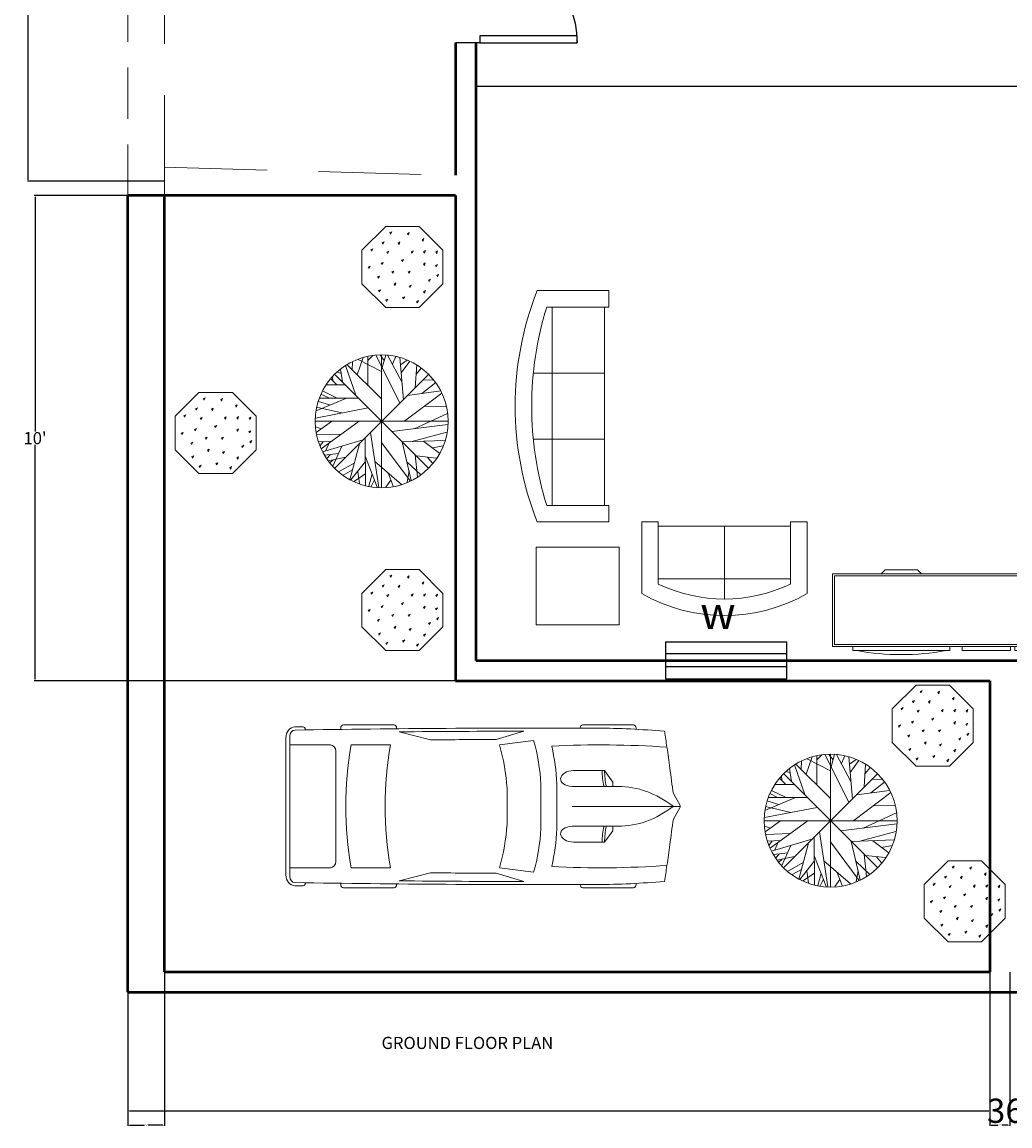
# Model space of a CAD drawing. Units: inches. Extents: x -10 to 557, y -66 to 886.
# Tile 1 of 6: x -3 to 241, y -66 to 207. Entities that reach past the tile are written whole.
import ezdxf

# ---------------------------------------------------------------- set-up
doc = ezdxf.new("R2010")
doc.units = ezdxf.units.IN
doc.header["$MEASUREMENT"] = 0
doc.linetypes.add('DASHED', pattern=[19.05, 12.7, -6.35])
for name, color, linetype, lineweight in [('A-ANNO-DIMS', 2, 'Continuous', 18), ('A-ANNO-TEXT', 7, 'Continuous', 18), ('A-DOOR', 4, 'Continuous', 25), ('A-EQPM', 9, 'Continuous', 18), ('A-FURN', 8, 'Continuous', 18), ('A-GLAZ', 4, 'Continuous', 25), ('A-WALL', 7, 'Continuous', 50), ('A-WALL-OVHD', 8, 'DASHED', 18), ('L-PLNT', 3, 'Continuous', 18)]:
    doc.layers.add(name, color=color, linetype=linetype, lineweight=lineweight)
doc.styles.get("Standard").update_dxf_attribs({"font": 'arial.ttf'})
doc.dimstyles.get("Standard").update_dxf_attribs({"dimtxt": 0.3, "dimasz": 0.4, "dimexe": 0.18, "dimexo": 0.0625, "dimgap": 0.09, "dimtad": 0, "dimtih": 1, "dimtoh": 1, "dimdec": 0, "dimrnd": 8, "dimzin": 0, "dimdsep": 46, "dimlunit": 3, "dimtxsty": 'Standard', "dimcen": 0.09, "dimadec": 0, "dimazin": 0, "dimtfac": 1, "dimtdec": 0, "dimtofl": 0, "dimtmove": 0, "dimatfit": 3, "dimfxl": 1, "dimtolj": 1, "dimtzin": 0, "dimarcsym": 0})

# ---------------------------------------------------------------- blocks, each defined once
blk = doc.blocks.new('*U33')
for p, q in [((0, 0), (0, -6)), ((24, 0), (24, -6))]:
    blk.add_line(p, q)
blk.add_lwpolyline([(0, 0), (0, 24), (1.75, 24), (1.75, 0)], close=True)
blk.add_arc((0, 0), 24, 0, 90)
blk = doc.blocks.new('Sofa - Roundback 7 ft.')
for p, q in [((-12.00002, -32.4421), (-12.00003, -6.5971)), ((11.99997, -32.4421), (11.99998, -6.5971)), ((-36.000027, -34), (-36.000027, -11.4696)), ((35.99998, -34), (35.99998, -11.4696)), ((-35.999844, -13.3819), (35.9998, -13.3819)), ((-36.000027, -32.4421), (35.99998, -32.4421))]:
    blk.add_line(p, q)
for points in [[(-36.000027, -34), (-42.000027, -34), (-42.000027, -8)], [(41.99998, -8), (41.99998, -34), (35.99998, -34)]]:
    blk.add_lwpolyline(points)
for centre, radius, start, end in [((0, -114.25), 114.25, 68.43141, 111.5686), ((-0.00001, -127.1968), 121.1968, 72.72033, 107.2797)]:
    blk.add_arc(centre, radius, start, end)
blk = doc.blocks.new('Sofa - Roundback Loveseat 5 ft.')
for p, q in [((0, -32.44198), (0, -5.99998)), ((-24, -33.99998), (-24, -11.46958)), ((24.00004, -33.99998), (24.00004, -11.46958)), ((-23.9998, -13.38178), (23.99986, -13.38178)), ((-24, -32.44198), (24.00004, -32.44198))]:
    blk.add_line(p, q)
for points in [[(-24, -33.99998), (-30, -33.99998), (-30, -7.99998)], [(30.00004, -7.99998), (30.00004, -33.99998), (24.00004, -33.99998)]]:
    blk.add_lwpolyline(points)
for centre, radius, start, end in [((0, -60.24998), 60.24998, 60.13715, 119.8628), ((0, -61.38438), 55.38444, 64.32083, 115.6792)]:
    blk.add_arc(centre, radius, start, end)
blk = doc.blocks.new('*U36')
for p, q in [((21.1, 37.41), (21.1, 36.83)), ((46.55, 38.89), (22.35, 38.89)), ((47.8, 37.39), (47.8, 37.41)), ((135.45, 37.07), (135.45, 37.41)), ((136.7, 38.89), (160.9, 38.89)), ((162.15, 37.41), (162.15, 36.77)), ((87.99, 31.87), (74.76, 35.92)), ((134.31, 35.6), (119.29, 31.78)), ((186.47, -33.5), (186.47, 33.5)), ((188.4, -32.76), (188.4, 32.76)), ((70.03, 31.54), (86.41, 29.35)), ((138.42, 29.35), (157.25, 29.35)), ((164.52, 26.39), (164.52, -26.39)), ((186.47, 29.35), (167.01, 29.35)), ((32.27, 11.63), (36.13, 17.17)), ((36.13, 17.17), (50.94, 17.17)), ((32.12, 9.51), (32.12, 11.15)), ((58.92, -10.77), (58.92, 10.77)), ((3.27, 6.13), (0.1, 0.41)), ((29.77, 9.51), (51.68, 9.51)), ((66.55, -10.53), (66.55, 10.53)), ((82.74, 8.5), (82.74, -8.5)), ((186.47, -10.53), (186.47, 10.53)), ((0, 0), (51.68, 0)), ((0.1, -0.41), (3.27, -6.13)), ((29.77, -9.51), (51.68, -9.51)), ((32.12, -9.51), (32.12, -11.15)), ((32.27, -11.63), (36.13, -17.17)), ((36.13, -17.17), (50.94, -17.17)), ((86.41, -29.35), (70.03, -31.54)), ((157.25, -29.35), (138.42, -29.35)), ((167.01, -29.35), (186.47, -29.35)), ((21.1, -37.41), (21.1, -36.83)), ((87.99, -31.87), (74.76, -35.92)), ((134.31, -35.6), (119.29, -31.78)), ((162.15, -37.41), (162.15, -36.77)), ((46.55, -38.89), (22.35, -38.89)), ((47.8, -37.39), (47.8, -37.41)), ((135.45, -37.07), (135.45, -37.41)), ((136.7, -38.89), (160.9, -38.89))]:
    blk.add_line(p, q)
for centre, major_axis, ratio, start_param, end_param in [((41.19, -490.86), (0, 528.23), 0.842304, 0.00281, 0.075598), ((22.35, 37.41), (0, -1.48), 0.842304, 3.141593, 4.712389), ((64.48, -10555.62), (0, 10593.03), 0.842304, -0.013397, 0.002797), ((46.55, 37.41), (0, 1.48), 0.842304, -1.570796, 0), ((136.7, 37.41), (0, -1.48), 0.842304, 3.141593, 4.712389), ((160.9, 37.41), (0, 1.48), 0.842304, -1.570796, 0), ((180.63, 35.84), (0, 2.22), 0.842304, -0.013017, 1.249894), ((64.48, -10556.36), (0, 10595.31), 0.842304, -0.013397, -0.013017), ((183.98, 32.76), (0, -5.25), 0.842304, 1.570796, 3.128196), ((266.03, -27.52), (0, 313.31), 0.842304, 1.367076, 1.39176), ((64.48, -10555.62), (0, -10591.55), 0.842304, 3.133765, 3.140441), ((95.79, -3666.35), (0, -3698.24), 0.842304, 3.134049, 3.144098), ((183.98, 33.5), (0, -2.96), 0.842304, 1.570796, 3.128196), ((259.18, -27.52), (0, -305.3), 0.842304, 4.528606, 4.561838), ((37.47, -593.96), (0, -623.33), 0.842304, 3.096046, 3.200911), ((134.4, 5.39), (0, -89.78), 0.842304, 4.449482, 4.652344), ((135.29, 5.39), (0, 81.77), 0.842304, 1.245306, 1.50788), ((149.6, 2.8), (0, -79.58), 0.842304, 4.372215, 4.640744), ((17.08, 0), (0, 147.02), 0.842304, 4.511394, 4.913384), ((35.91, 0), (0, 147.02), 0.842304, 4.511394, 4.913384), ((167.01, 26.39), (0, 2.96), 0.842304, 0, 1.570796), ((-204.49, 52.4), (0, -250.96), 0.842304, 1.385369, 1.434372), ((13.04, 17.01), (0, 27.42), 0.842304, 4.435146, 4.718221), ((14.2, 17.01), (0, 27.42), 0.842304, 4.435146, 4.718221), ((50.79, 13.34), (6.34, -0.36), 0.603834, -1.395552, 1.581315), ((32.75, 11.15), (0, 0.74), 0.842304, 0.879714, 1.570796), ((29.77, -46.66), (0, 56.17), 0.842304, 0, 0.590319), ((0.62, 0), (0, -0.74), 0.842304, 4.131459, 5.293319), ((29.77, 46.66), (0, 56.17), 0.842304, 2.551274, 3.141593), ((-204.49, -52.4), (0, 250.96), 0.842304, -1.434372, -1.385369), ((13.04, -17.01), (0, -27.42), 0.842304, 1.564964, 1.848039), ((14.2, -17.01), (0, -27.42), 0.842304, 1.564964, 1.848039), ((135.29, -5.39), (0, -81.77), 0.842304, -1.50788, -1.245306), ((149.6, -2.8), (0, -79.58), 0.842304, -1.499151, -1.230623), ((32.75, -11.15), (0, -0.74), 0.842304, 4.712389, 5.403472), ((134.4, -5.39), (0, -89.78), 0.842304, -1.510751, -1.307889), ((259.18, 27.52), (0, 305.3), 0.842304, 1.721348, 1.754579), ((266.03, 27.52), (0, 313.31), 0.842304, 1.749832, 1.774517), ((37.47, 593.96), (0, -623.33), 0.842304, -0.059319, 0.045547), ((167.01, -26.39), (0, -2.96), 0.842304, 4.712389, 6.283185), ((41.19, 490.86), (0, -528.23), 0.842304, -0.075598, -0.00281), ((64.48, 10555.62), (0, 10593.03), 0.842304, 3.138796, 3.15499), ((64.48, 10555.62), (0, -10591.55), 0.842304, 0.001152, 0.007828), ((95.79, 3666.35), (0, -3698.24), 0.842304, -0.002505, 0.007544), ((180.63, -35.84), (0, -2.22), 0.842304, -1.249894, 0.013017), ((183.98, -33.5), (0, 2.96), 0.842304, 3.15499, 4.712389), ((183.98, -32.76), (0, -5.25), 0.842304, 0.013397, 1.570796), ((22.35, -37.41), (0, 1.48), 0.842304, 1.570796, 3.141593), ((46.55, -37.41), (0, -1.48), 0.842304, 0, 1.570796), ((136.7, -37.41), (0, -1.48), 0.842304, -1.570796, 0), ((160.9, -37.41), (0, 1.48), 0.842304, 3.141593, 4.712389), ((64.48, 10556.36), (0, 10595.31), 0.842304, 3.15461, 3.15499)]:
    blk.add_ellipse(centre, major_axis=major_axis, ratio=ratio, start_param=start_param, end_param=end_param)
at = {"extrusion": (0, 0, -1)}
blk.add_ellipse((50.79, -13.34), major_axis=(6.34, 0.36), ratio=0.603834, start_param=-1.395552, end_param=1.581315, dxfattribs=at)
blk = doc.blocks.new('*D42')
at = {"layer": 'A-ANNO-DIMS', "color": 0, "lineweight": -2, "ltscale": 2, "transparency": 16777216}
for p, q in [((31.91, 265.32), (-1.86, 265.32)), ((-1.68, 264.92), (-1.68, 218.2)), ((-1.68, 168.23), (-1.68, 214.95)), ((31.91, 167.83), (-1.86, 167.83))]:
    blk.add_line(p, q, dxfattribs=at)
at = {"layer": 'A-ANNO-DIMS', "color": 0, "ltscale": 2, "transparency": 16777216}
for points in [[(-1.75, 264.92), (-1.61, 264.92), (-1.68, 265.32)], [(-1.75, 168.23), (-1.61, 168.23), (-1.68, 167.83)]]:
    blk.add_solid(points, dxfattribs=at)
at = {"layer": 'Defpoints', "color": 0, "ltscale": 2, "transparency": 16777216}
for p in [(31.97, 265.32), (-1.68, 167.83), (31.97, 167.83)]:
    blk.add_point(p, dxfattribs=at)
at = {"layer": 'A-ANNO-DIMS', "color": 0, "ltscale": 2, "transparency": 16777216, "insert": (-1.68, 216.57), "char_height": 0.3, "attachment_point": 5}
blk.add_mtext("\\A1;{\\H10x;8'}", dxfattribs=at)
blk = doc.blocks.new('*D43')
at = {"layer": 'A-ANNO-DIMS', "color": 0, "lineweight": -2, "ltscale": 2, "transparency": 16777216}
for p, q in [((103.91, 164.32), (-0.17, 164.32)), ((0.01, 163.92), (0.01, 105.94)), ((0.01, 44.72), (0.01, 102.7)), ((103.91, 44.32), (-0.17, 44.32))]:
    blk.add_line(p, q, dxfattribs=at)
at = {"layer": 'A-ANNO-DIMS', "color": 0, "ltscale": 2, "transparency": 16777216}
for points in [[(-0.06, 163.92), (0.08, 163.92), (0.01, 164.32)], [(-0.06, 44.72), (0.08, 44.72), (0.01, 44.32)]]:
    blk.add_solid(points, dxfattribs=at)
at = {"layer": 'Defpoints', "color": 0, "ltscale": 2, "transparency": 16777216}
for p in [(103.97, 164.32), (0.01, 44.32), (103.97, 44.32)]:
    blk.add_point(p, dxfattribs=at)
at = {"layer": 'A-ANNO-DIMS', "color": 0, "ltscale": 2, "transparency": 16777216, "insert": (0.01, 104.32), "char_height": 0.3, "attachment_point": 5}
blk.add_mtext("\\A1;{\\H10x;10'}", dxfattribs=at)
blk = doc.blocks.new('*D49')
at = {"layer": 'A-ANNO-DIMS', "color": 0, "lineweight": -2, "ltscale": 2, "transparency": 16777216}
for p, q in [((108.97, 177.7), (108.97, 191.53)), ((109.37, 191.35), (274.2, 191.35)), ((449.57, 191.35), (284.74, 191.35)), ((449.97, 177.7), (449.97, 191.53))]:
    blk.add_line(p, q, dxfattribs=at)
at = {"layer": 'A-ANNO-DIMS', "color": 0, "ltscale": 2, "transparency": 16777216}
for points in [[(109.37, 191.42), (109.37, 191.28), (108.97, 191.35)], [(449.57, 191.42), (449.57, 191.28), (449.97, 191.35)]]:
    blk.add_solid(points, dxfattribs=at)
at = {"layer": 'Defpoints', "color": 0, "ltscale": 2, "transparency": 16777216}
for p in [(449.97, 191.35), (108.97, 177.64), (449.97, 177.64)]:
    blk.add_point(p, dxfattribs=at)
at = {"layer": 'A-ANNO-DIMS', "color": 0, "ltscale": 2, "transparency": 16777216, "insert": (279.47, 191.35), "char_height": 0.3, "attachment_point": 5}
blk.add_mtext('\\A1;{\\H10x;28\'-8"}', dxfattribs=at)
blk = doc.blocks.new('Stepping Stone - hexagonal')
for p, q in [((-5.1, 10.07), (-10.96, 4.2)), ((3.2, 10.07), (-5.1, 10.07)), ((-3.56, 8.74), (-4.06, 8.54)), ((-4.06, 8.54), (-3.91, 8.2)), ((-3.91, 8.2), (-3.56, 8.74)), ((0.7, 8.56), (0.27, 8.26)), ((0.27, 8.26), (0.5, 7.96)), ((0.5, 7.96), (0.7, 8.56)), ((9.06, 4.2), (3.2, 10.07)), ((-5.45, 6.27), (-5.95, 6.07)), ((-5.95, 6.07), (-5.79, 5.73)), ((-5.79, 5.73), (-5.45, 6.27)), ((-1.57, 6.24), (-2, 5.93)), ((-2, 5.93), (-1.77, 5.63)), ((-1.77, 5.63), (-1.57, 6.24)), ((4.33, 7.05), (3.9, 6.74)), ((3.9, 6.74), (4.13, 6.45)), ((4.13, 6.45), (4.33, 7.05)), ((-10.96, 4.2), (-10.96, -4.09)), ((-8.31, 4.52), (-8.81, 4.32)), ((-8.81, 4.32), (-8.65, 3.98)), ((-8.65, 3.98), (-8.31, 4.52)), ((-4.32, 3.92), (-4.82, 3.72)), ((-4.82, 3.72), (-4.67, 3.38)), ((-4.67, 3.38), (-4.32, 3.92)), ((1.65, 4.08), (1.22, 3.77)), ((1.22, 3.77), (1.45, 3.48)), ((1.45, 3.48), (1.65, 4.08)), ((4.71, 4.1), (4.27, 3.8)), ((4.27, 3.8), (4.5, 3.5)), ((4.5, 3.5), (4.71, 4.1)), ((7.74, 4.01), (7.3, 3.7)), ((7.3, 3.7), (7.53, 3.41)), ((7.53, 3.41), (7.74, 4.01)), ((9.06, -4.09), (9.06, 4.2)), ((-8.97, 0.22), (-9.47, 0.02)), ((-9.47, 0.02), (-9.31, -0.32)), ((-9.31, -0.32), (-8.97, 0.22)), ((-5.72, 1.16), (-6.22, 0.96)), ((-6.22, 0.96), (-6.07, 0.63)), ((-6.07, 0.63), (-5.72, 1.16)), ((-0.72, 1.92), (-1.22, 1.73)), ((-1.22, 1.73), (-1.07, 1.39)), ((-1.07, 1.39), (-0.72, 1.92)), ((4.67, 1.05), (4.23, 0.74)), ((4.23, 0.74), (4.46, 0.44)), ((4.46, 0.44), (4.67, 1.05)), ((7.72, 0.63), (7.23, 0.43)), ((7.23, 0.43), (7.38, 0.09)), ((7.38, 0.09), (7.72, 0.63)), ((-6.63, -2.22), (-7.13, -2.42)), ((-7.13, -2.42), (-6.97, -2.76)), ((-6.97, -2.76), (-6.63, -2.22)), ((-3.1, -0.96), (-3.6, -1.16)), ((-3.6, -1.16), (-3.44, -1.5)), ((-3.44, -1.5), (-3.1, -0.96)), ((0.94, -0.97), (0.45, -1.17)), ((0.45, -1.17), (0.6, -1.51)), ((0.6, -1.51), (0.94, -0.97)), ((7.94, -1.78), (7.5, -2.09)), ((7.5, -2.09), (7.73, -2.38)), ((7.73, -2.38), (7.94, -1.78)), ((-10.96, -4.09), (-5.1, -9.96)), ((-2.57, -3.91), (-3, -4.22)), ((-3, -4.22), (-2.77, -4.51)), ((-2.77, -4.51), (-2.57, -3.91)), ((1.22, -4.48), (0.72, -4.68)), ((0.72, -4.68), (0.88, -5.02)), ((0.88, -5.02), (1.22, -4.48)), ((3.2, -9.96), (9.06, -4.09)), ((5.96, -2.99), (5.47, -3.18)), ((5.47, -3.18), (5.62, -3.52)), ((5.62, -3.52), (5.96, -2.99)), ((-6.38, -5.59), (-6.87, -5.79)), ((-6.87, -5.79), (-6.72, -6.13)), ((-6.72, -6.13), (-6.38, -5.59)), ((-4.59, -7.91), (-5.08, -8.11)), ((-5.08, -8.11), (-4.93, -8.45)), ((-4.93, -8.45), (-4.59, -7.91)), ((-0.41, -7.32), (-0.91, -7.51)), ((-0.91, -7.51), (-0.76, -7.85)), ((-0.76, -7.85), (-0.41, -7.32)), ((4.7, -5.8), (4.26, -6.11)), ((4.26, -6.11), (4.49, -6.4)), ((4.49, -6.4), (4.7, -5.8)), ((-5.1, -9.96), (3.2, -9.96)), ((2.97, -8.26), (2.54, -8.57)), ((2.54, -8.57), (2.77, -8.86)), ((2.77, -8.86), (2.97, -8.26))]:
    blk.add_line(p, q)
blk = doc.blocks.new('Tree - deciduous plan')
for p, q in [((2.426, 54.9406), (-1.4472, 59.9056)), ((0, 59.9996), (0, -60)), ((-32.6092, 50.4264), (-23.2782, 23.5674)), ((-31.2008, 51.1035), (-0.2149, 20.1818)), ((-26.4472, 46.5894), (-26.2712, 53.8116)), ((-22.0458, 42.0753), (-16.5881, 57.6486)), ((-21.1656, 55.8436), (-0.0388, 45.0094)), ((-12.5388, 54.9406), (-7.9613, 59.4546)), ((-12.3627, 32.1443), (-12.5388, 58.7776)), ((-5.3205, 59.6806), (16.5105, 16.7963)), ((0.4894, 48.6208), (3.6584, 59.6806)), ((18.2711, 35.5298), (5.419, 59.6806)), ((9.8203, 51.5549), (12.8133, 58.5516)), ((19.6795, 19.5047), (16.3344, 57.6486)), ((17.0387, 51.1035), (23.2006, 55.1666)), ((17.7429, 43.6552), (25.4894, 54.2636)), ((31.6513, 50.8778), (30.2429, 30.5643)), ((-43.8768, 36.4326), (-44.405, 40.2696)), ((42, 42), (-42, -42)), ((42, -42), (-42, 42)), ((-40.1797, 44.558), (-36.4825, 43.2038)), ((-37.0107, 47.0408), (-35.25, 35.5298)), ((31.1232, 42.5267), (35.8767, 48.1693)), ((-49.8627, 32.8214), (-32.7853, 32.8214)), ((-45.8134, 38.2383), (-40.5318, 33.0471)), ((36.2288, 25.1474), (48.9049, 35.0784)), ((37.1091, 37.1098), (46.6161, 37.5612)), ((-32.2571, 20.6333), (-59.1937, 9.348)), ((-56.0247, 20.859), (-20.8134, 20.859)), ((-54.7923, 24.4702), (-47.75, 21.0847)), ((-53.2078, 27.4044), (-40.1797, 20.859)), ((54.3626, 25.3731), (20.9119, 0.3198)), ((23.3767, 23.3417), (53.3063, 27.4044)), ((-59.7219, 2.8025), (-12.0106, 12.0565)), ((-58.6656, 12.7336), (-35.9543, 7.5424)), ((-57.081, 17.9248), (-47.0458, 14.7649)), ((38.5175, 13.4107), (58.2359, 13.6364)), ((-54.6162, -24.7335), (-20.2853, 0.0941)), ((29.3626, -6.6771), (59.4682, 7.091)), ((-60, 0), (60, 0)), ((-59.7219, -4.8714), (-54.2641, -6.6771)), ((-45.2853, -0.1316), (-59.0177, -10.0627)), ((9.2922, -9.1598), (59.6443, -2.8401)), ((26.3697, -18.4138), (58.9401, -9.8369)), ((-58.4895, -12.3197), (-36.4825, -11.6426)), ((-57.081, -18.4138), (-45.2853, -17.9624)), ((-52.6797, -18.188), (-55.4966, -22.0251)), ((-53.2078, -27.442), (-16.7641, -16.6081)), ((-47.2219, -19.3166), (-50.2148, -26.3135)), ((-14.8275, -15.0282), (-14.6515, -57.6865)), ((-10.074, -10.0627), (-2.5036, -59.7178)), ((-0.0388, -19.0909), (25.8415, -53.8495)), ((18.6232, -18.6394), (26.7218, -53.3981)), ((18.7992, -18.6394), (57.3556, -17.2853)), ((38.1654, -18.188), (52.426, -29.0219)), ((-38.9472, -29.0219), (-51.4472, -30.6018)), ((-35.9543, -22.4765), (-44.0529, -40.5329)), ((-19.9331, -20.2194), (-28.5599, -52.721)), ((45.9119, -24.0564), (55.595, -22.2508)), ((-46.5177, -30.1504), (-49.5106, -33.536)), ((-32.4331, -32.4075), (-48.1021, -35.5674)), ((-43.7008, -34.6645), (-46.6937, -37.373)), ((-24.6867, -37.8244), (-38.7712, -45.7241)), ((-14.6515, -36.2445), (-27.6797, -52.9467)), ((-14.6515, -32.1818), (-3.912, -59.4922)), ((-6.2008, -36.2445), (17.919, -57.0094)), ((22.8485, -36.4702), (35.3485, -48.4326)), ((30.419, -30.1504), (32.3556, -50.0125)), ((31.4753, -31.279), (49.6091, -33.3103)), ((41.5105, -32.6332), (46.088, -38.0501)), ((-26.2712, -43.9185), (-34.7219, -48.6583)), ((-14.6515, -47.3041), (-25.0388, -54.3009)), ((-21.5177, -45.4984), (-19.9331, -56.1065)), ((-8.4895, -47.5298), (-11.4825, -58.5893)), ((5.9471, -46.6269), (10.5246, -58.5893)), ((24.7852, -44.8213), (23.0246, -54.978)), ((-6.3768, -52.721), (-9.3698, -58.815)), ((8.4119, -53.1724), (3.8344, -59.4922))]:
    blk.add_line(p, q)
blk.add_circle((0, 0), 60)
blk = doc.blocks.new('Entertainment Center')
for p, q in [((-4, 0), (-5, -1)), ((4, 0), (-4, 0)), ((5, -1), (4, 0)), ((-17, -19), (-17, -1)), ((-17, -1), (43, -1)), ((-16.5, -18.5), (-16.5, -1.5)), ((-16.5, -1.5), (42.5, -1.5)), ((42.5, -1.5), (42.5, -18.5)), ((43, -1), (43, -19)), ((43, -19), (-17, -19)), ((42.5, -18.5), (-16.5, -18.5)), ((-12, -20), (-12, -19)), ((12, -19), (12, -20)), ((15, -20), (15, -19)), ((27, -19), (27, -20)), ((28, -20), (28, -19)), ((40, -19), (40, -20)), ((12, -20), (-12, -20)), ((27, -20), (15, -20)), ((40, -20), (28, -20))]:
    blk.add_line(p, q)
blk.add_arc((0, 40), 61, 259.6111, 280.3889)
blk = doc.blocks.new('*D53')
at = {"layer": 'A-ANNO-DIMS', "color": 0, "lineweight": -2, "ltscale": 2, "transparency": 16777216}
for p, q in [((22.97, -32.74), (22.97, -62.2)), ((458.97, -31.14), (458.97, -62.2)), ((23.37, -62.02), (235.79, -62.02)), ((458.57, -62.02), (246.15, -62.02))]:
    blk.add_line(p, q, dxfattribs=at)
at = {"layer": 'A-ANNO-DIMS', "color": 0, "ltscale": 2, "transparency": 16777216}
for points in [[(23.37, -61.96), (23.37, -62.09), (22.97, -62.02)], [(458.57, -61.96), (458.57, -62.09), (458.97, -62.02)]]:
    blk.add_solid(points, dxfattribs=at)
at = {"layer": 'Defpoints', "color": 0, "ltscale": 2, "transparency": 16777216}
for p in [(22.97, -32.68), (458.97, -31.08), (458.97, -62.02)]:
    blk.add_point(p, dxfattribs=at)
at = {"layer": 'A-ANNO-DIMS', "color": 0, "ltscale": 2, "transparency": 16777216, "insert": (240.97, -62.02), "char_height": 0.3, "attachment_point": 5}
blk.add_mtext("\\A1;{\\H20x;36'}", dxfattribs=at)
blk = doc.blocks.new('WIN-900')
for p, q in [((0, 6.25), (30, 6.25)), ((0, 4.5), (30, 4.5)), ((0, 3.05), (30, 3.05))]:
    blk.add_line(p, q)
blk.add_lwpolyline([(0, 9), (0, 0), (30, 0), (30, 9)], close=True)
blk = doc.blocks.new('*D83')
at = {"layer": 'A-ANNO-DIMS', "color": 0, "lineweight": -2, "ltscale": 2, "transparency": 16777216}
for p, q in [((31.97, -27.74), (31.97, -65.76)), ((22.97, -32.74), (22.97, -65.76)), ((23.37, -65.58), (26.98, -65.58)), ((31.57, -65.58), (27.96, -65.58))]:
    blk.add_line(p, q, dxfattribs=at)
at = {"layer": 'A-ANNO-DIMS', "color": 0, "ltscale": 2, "transparency": 16777216}
for points in [[(23.37, -65.51), (23.37, -65.64), (22.97, -65.58)], [(31.57, -65.51), (31.57, -65.64), (31.97, -65.58)]]:
    blk.add_solid(points, dxfattribs=at)
at = {"layer": 'Defpoints', "color": 0, "ltscale": 2, "transparency": 16777216}
for p in [(31.97, -27.68), (22.97, -32.68), (31.97, -65.58)]:
    blk.add_point(p, dxfattribs=at)
at = {"layer": 'A-ANNO-DIMS', "color": 0, "ltscale": 2, "transparency": 16777216, "insert": (27.47, -65.58), "char_height": 0.3, "attachment_point": 5}
blk.add_mtext('\\A1;0\'-9"', dxfattribs=at)
blk = doc.blocks.new('*D84')
at = {"layer": 'A-ANNO-DIMS', "color": 0, "lineweight": -2, "ltscale": 2, "transparency": 16777216}
for p, q in [((235.97, -27.74), (235.97, -65.76)), ((240.97, -27.74), (240.97, -65.76)), ((236.37, -65.58), (237.98, -65.58)), ((240.57, -65.58), (238.96, -65.58))]:
    blk.add_line(p, q, dxfattribs=at)
at = {"layer": 'A-ANNO-DIMS', "color": 0, "ltscale": 2, "transparency": 16777216}
for points in [[(236.37, -65.51), (236.37, -65.64), (235.97, -65.58)], [(240.57, -65.51), (240.57, -65.64), (240.97, -65.58)]]:
    blk.add_solid(points, dxfattribs=at)
at = {"layer": 'Defpoints', "color": 0, "ltscale": 2, "transparency": 16777216}
for p in [(235.97, -27.68), (240.97, -27.68), (240.97, -65.58)]:
    blk.add_point(p, dxfattribs=at)
at = {"layer": 'A-ANNO-DIMS', "color": 0, "ltscale": 2, "transparency": 16777216, "insert": (238.47, -65.58), "char_height": 0.3, "attachment_point": 5}
blk.add_mtext('\\A1;0\'-5"', dxfattribs=at)

msp = doc.modelspace()

# ---------------------------------------------------------------- linework, layer by layer
at = {"layer": 'A-FURN'}
msp.add_lwpolyline([(123.83, 77.39), (144.39, 77.39), (144.39, 58.13), (123.83, 58.13)], close=True, dxfattribs=at)
at = {"layer": 'A-WALL'}
for p, q in [((103.97, 202.08), (103.97, 169.32)), ((108.97, 202.08), (108.97, 49.32)), ((103.97, 164.32), (22.97, 164.32)), ((22.97, -32.68), (22.97, 164.26)), ((31.97, -27.68), (31.97, 164.32)), ((103.97, 164.32), (103.97, 44.32)), ((108.97, 49.32), (276.97, 49.32)), ((103.97, 44.32), (235.97, 44.32)), ((235.97, 44.32), (235.97, -27.68)), ((31.97, -27.68), (235.97, -27.68)), ((22.97, -32.68), (458.97, -32.68))]:
    msp.add_line(p, q, dxfattribs=at)
at = {"layer": 'A-WALL-OVHD'}
msp.add_line((22.97, 164.26), (22.97, 265.28), dxfattribs=at)
at = {"layer": 'A-WALL-OVHD', "ltscale": 2}
for p, q in [((31.97, 265.32), (31.97, 164.32)), ((31.97, 164.32), (31.97, 171.33)), ((31.97, 171.33), (103.97, 169.32))]:
    msp.add_line(p, q, dxfattribs=at)

# ---------------------------------------------------------------- block references
at = {"layer": 'A-DOOR', "xscale": -1, "rotation": 270}
msp.add_blockref('*U33', (109.97, 202.08), dxfattribs=at)
at = {"layer": 'A-EQPM', "xscale": -0.51745172860646, "yscale": 0.51745172860646, "zscale": 0.51745172860646}
msp.add_blockref('*U36', (159.48, 13.26), dxfattribs=at)
at = {"layer": 'A-FURN', "xscale": 0.6812959275706195, "yscale": 0.6812959275706195, "zscale": 0.6812959275706195}
for name, p, rotation in [('Sofa - Roundback 7 ft.', (118.68, 112.21), 90), ('Sofa - Roundback Loveseat 5 ft.', (170.4, 60.43), 180)]:
    msp.add_blockref(name, p, dxfattribs=dict(at, rotation=rotation))
at = {"layer": 'A-FURN'}
msp.add_blockref('Entertainment Center', (214.15, 71.78), dxfattribs=at)
at = {"layer": 'A-GLAZ'}
msp.add_blockref('WIN-900', (155.82, 44.82), dxfattribs=at)
at = {"layer": 'L-PLNT', "ltscale": 2}
for p in [(91.78, 146.6), (45.62, 105.53), (91.78, 61.73), (222.86, 33.16), (230.77, -10.27)]:
    msp.add_blockref('Stepping Stone - hexagonal', p, dxfattribs=at)
at = {"layer": 'L-PLNT', "ltscale": 2, "xscale": 0.2739233807933292, "yscale": 0.2739233807933292, "zscale": 0.2739233807933292}
for p in [(85.67, 108.48), (196.64, 9.7)]:
    msp.add_blockref('Tree - deciduous plan', p, dxfattribs=at)

# ---------------------------------------------------------------- texts
at = {"layer": 'A-ANNO-TEXT', "insert": (164.42, 65.13), "char_height": 8, "attachment_point": 1}
msp.add_mtext_dynamic_manual_height_columns('w', width=13.506, gutter_width=1, heights=[0], dxfattribs=at)
at = {"layer": 'A-ANNO-TEXT', "ltscale": 2, "insert": (85.65, -43.75), "char_height": 3, "attachment_point": 1}
msp.add_mtext_dynamic_manual_height_columns('GROUND FLOOR PLAN ', width=164.3173, gutter_width=1, heights=[0], dxfattribs=at)

# ---------------------------------------------------------------- dimensions: what is measured, and where the dimension line sits
at = {"layer": 'A-ANNO-DIMS', "ltscale": 2}
for base, p1, p2, picture, middle in [((-1.68, 167.83), (31.97, 265.32), (31.97, 167.83), '*D42', (-1.68, 216.57)), ((0.01, 44.32), (103.97, 164.32), (103.97, 44.32), '*D43', (0.01, 104.32))]:
    dim = msp.add_linear_dim(base=base, p1=p1, p2=p2, angle=90, text='{\\H10x;<>}', dimstyle='Standard', override={"dimclrd": 0, "dimclre": 0, "dimclrt": 0}, dxfattribs=at)
    dim.commit()
    dim.dimension.update_dxf_attribs({"geometry": picture, "text_midpoint": middle})
for base, p1, p2, text, picture, middle in [((449.97, 191.35), (108.97, 177.64), (449.97, 177.64), '{\\H10x;<>}', '*D49', (279.47, 191.35)), ((458.97, -62.02), (22.97, -32.68), (458.97, -31.08), '{\\H20x;<>}', '*D53', (240.97, -62.02))]:
    dim = msp.add_linear_dim(base=base, p1=p1, p2=p2, text=text, dimstyle='Standard', override={"dimclrd": 0, "dimclre": 0, "dimclrt": 0}, dxfattribs=at)
    dim.commit()
    dim.dimension.update_dxf_attribs({"geometry": picture, "text_midpoint": middle})
for base, p1, p2, picture, middle in [((31.97, -65.58), (22.97, -32.68), (31.97, -27.68), '*D83', (27.47, -65.58)), ((240.97, -65.58), (235.97, -27.68), (240.97, -27.68), '*D84', (238.47, -65.58))]:
    dim = msp.add_linear_dim(base=base, p1=p1, p2=p2, dimstyle='Standard', override={"dimdec": 1, "dimlfac": 1, "dimrnd": 0, "dimzin": 1, "dimdsep": 46, "dimlunit": 4, "dimfrac": 2}, dxfattribs=at)
    dim.commit()
    dim.dimension.update_dxf_attribs({"geometry": picture, "text_midpoint": middle})

doc.saveas('drawing.dxf')
